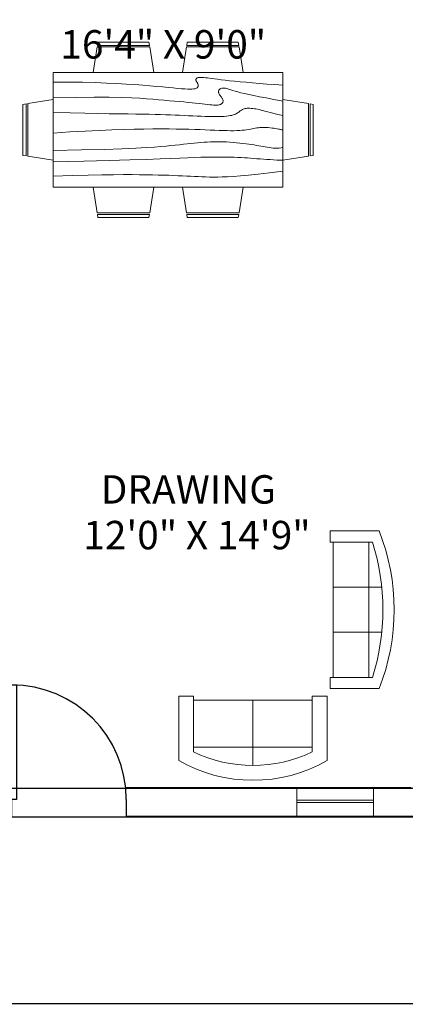
# Model space of a CAD drawing. Units: inches. Extents: x -46 to 1145, y -527 to 760.
# Tile 18 of 57: x 788 to 909, y -527 to -218. Entities that reach past the tile are written whole.
import ezdxf

# ---------------------------------------------------------------- set-up
doc = ezdxf.new("R2010")
doc.units = ezdxf.units.IN
doc.header["$MEASUREMENT"] = 0
for name, color, linetype, lineweight in [('A-ANNO-DIMS', 2, 'Continuous', 18), ('A-AREA-IDEN', 1, 'Continuous', 18), ('A-FURN', 2, 'Continuous', 13), ('C-SITE', 7, 'Continuous', 30), ('DOORS', 3, 'Continuous', 25), ('WALLS', 4, 'Continuous', 40), ('WINDOWS', 240, 'Continuous', 20)]:
    doc.layers.add(name, color=color, linetype=linetype, lineweight=lineweight)
doc.styles.get("Standard").update_dxf_attribs({"font": 'arial.ttf'})
doc.dimstyles.get("Standard").update_dxf_attribs({"dimtxt": 0.18, "dimasz": 0.18, "dimexe": 0.18, "dimexo": 0.0625, "dimgap": 0.09, "dimtad": 0, "dimtih": 1, "dimtoh": 1, "dimdec": 0, "dimzin": 0, "dimdsep": 46, "dimlunit": 3, "dimtxsty": 'Standard', "dimcen": 0.09, "dimadec": 0, "dimazin": 0, "dimtfac": 1, "dimtdec": 0, "dimtofl": 0, "dimtmove": 0, "dimatfit": 3, "dimfxl": 1, "dimtolj": 1, "dimtzin": 0, "dimarcsym": 0})

# ---------------------------------------------------------------- blocks, each defined once
blk = doc.blocks.new('Dining Set - 36 x 72 in.')
for p, q in [((-22.2343, 26.00059), (-23.4847, 17.99762)), ((-22.2304, 26), (-5.7608, 26)), ((-22, 27.5), (-22.1562, 26.50042)), ((-5.8416, 26.5), (-22.1534, 26.5)), ((-22, 27.5), (-6, 27.5)), ((-5.8437, 26.49966), (-6, 27.5)), ((-4.5152, 17.99762), (-5.7655, 25.99926)), ((5.7657, 26.00059), (4.5153, 17.99762)), ((5.7696, 26), (22.2392, 26)), ((6, 27.5), (5.8438, 26.50042)), ((22.1584, 26.5), (5.8466, 26.5)), ((6, 27.5), (22, 27.5)), ((22.1563, 26.49966), (22, 27.5)), ((23.4848, 17.99762), (22.2345, 25.99926)), ((36, 18), (-36, 18)), ((-36, 18), (-36, -18)), ((36, -18), (36, 18)), ((-44.0006, 8.23428), (-35.9976, 9.48474)), ((44.0006, 8.23428), (35.9976, 9.48474)), ((-45.5, 8), (-44.5004, 8.15617)), ((-45.5, 8), (-45.5, -8)), ((-44.5, -8.15843), (-44.5, 8.15338)), ((-44, 8.23041), (-44, -8.23915)), ((44, 8.23041), (44, -8.23915)), ((44.5, -8.15843), (44.5, 8.15338)), ((45.5, 8), (44.5005, 8.15617)), ((45.5, 8), (45.5, -8)), ((-44.4997, -8.15631), (-45.5, -8)), ((-35.9976, -9.48476), (-43.9993, -8.2345)), ((35.9976, -9.48476), (43.9993, -8.2345)), ((44.4997, -8.15631), (45.5, -8)), ((-36, -18), (36, -18)), ((-22.2343, -26.0006), (-23.4847, -17.99762)), ((-4.5152, -17.99762), (-5.7655, -25.99928)), ((5.7657, -26.0006), (4.5153, -17.99762)), ((23.4848, -17.99762), (22.2345, -25.99928)), ((-22.2304, -26), (-5.7608, -26)), ((-22, -27.5), (-22.1562, -26.50044)), ((-5.8416, -26.5), (-22.1534, -26.5)), ((-22, -27.5), (-6, -27.5)), ((-5.8437, -26.49967), (-6, -27.5)), ((5.7696, -26), (22.2392, -26)), ((6, -27.5), (5.8438, -26.50044)), ((22.1584, -26.5), (5.8466, -26.5)), ((6, -27.5), (22, -27.5)), ((22.1563, -26.49967), (22, -27.5))]:
    blk.add_line(p, q)
for points in [[(-36, 15), (-31.1772, 14.97754), (-26.8079, 14.91406), (-22.8538, 14.81543), (-19.276, 14.6875), (-16.0362, 14.53613), (-13.0957, 14.36718), (-10.4159, 14.18652), (-7.9583, 14), (-5.6904, 13.81315), (-3.6035, 13.63021), (-1.6954, 13.45508), (0.0365, 13.29166), (1.5945, 13.14388), (2.9811, 13.01562), (4.1988, 12.9108), (5.25, 12.83333), (6.1393, 12.78613), (6.8802, 12.76823), (7.4883, 12.77767), (7.9792, 12.8125), (8.3685, 12.87077), (8.6719, 12.95052), (8.9049, 13.0498), (9.0833, 13.16666), (9.2205, 13.29899), (9.3216, 13.44401), (9.3895, 13.59879), (9.4271, 13.76041), (9.4373, 13.92594), (9.4232, 14.09245), (9.3875, 14.257), (9.3333, 14.41666), (9.2638, 14.56917), (9.1836, 14.71484), (9.0975, 14.85465), (9.0104, 14.98958), (8.9272, 15.1206), (8.8529, 15.2487), (8.7922, 15.37483), (8.75, 15.5), (8.7305, 15.62467), (8.7344, 15.74739), (8.7617, 15.86621), (8.8125, 15.97916), (8.8867, 16.08431), (8.9844, 16.17968), (9.1055, 16.26334), (9.25, 16.33333), (9.4189, 16.38802), (9.6172, 16.42708), (9.8506, 16.45052), (10.125, 16.45833), (10.4463, 16.45052), (10.8203, 16.42708), (11.2529, 16.38802), (11.75, 16.33333), (12.3184, 16.26318), (12.9694, 16.17838), (13.7151, 16.07991), (14.5677, 15.96875), (15.5395, 15.84586), (16.6426, 15.71224), (17.8893, 15.56884), (19.2917, 15.41666), (20.859, 15.25667), (22.5879, 15.08984), (24.4721, 14.91715), (26.5052, 14.73958), (28.6809, 14.5581), (30.9929, 14.3737), (33.4347, 14.18733), (36, 14)], [(-36, 10), (-28.9766, 10.14274), (-23.1725, 10.20442), (-18.4241, 10.19775), (-14.5677, 10.13541), (-11.4399, 10.03011), (-8.877, 9.89453), (-6.7154, 9.74137), (-4.7917, 9.58333), (-2.9698, 9.43082), (-1.2246, 9.28515), (0.4415, 9.14534), (2.026, 9.01041), (3.5266, 8.87939), (4.9408, 8.7513), (6.266, 8.62516), (7.5, 8.5), (8.6411, 8.37549), (9.6914, 8.2539), (10.6538, 8.13818), (11.5312, 8.03125), (12.3267, 7.93603), (13.043, 7.85547), (13.6831, 7.79248), (14.25, 7.75), (14.7471, 7.7303), (15.1797, 7.73307), (15.5537, 7.75732), (15.875, 7.80208), (16.1494, 7.86637), (16.3828, 7.94922), (16.5811, 8.04964), (16.75, 8.16666), (16.8944, 8.29915), (17.0143, 8.44531), (17.1089, 8.60319), (17.1771, 8.77083), (17.218, 8.94629), (17.2305, 9.1276), (17.2137, 9.31282), (17.1667, 9.5), (17.0895, 9.6875), (16.987, 9.875), (16.8649, 10.0625), (16.7292, 10.25), (16.5856, 10.4375), (16.4401, 10.625), (16.2985, 10.8125), (16.1667, 11), (16.05, 11.18733), (15.9518, 11.3737), (15.8752, 11.5581), (15.8229, 11.73958), (15.798, 11.91715), (15.8034, 12.08984), (15.842, 12.25667), (15.9167, 12.41666), (16.0295, 12.56836), (16.1784, 12.70833), (16.3605, 12.83268), (16.5729, 12.9375), (16.8127, 13.01888), (17.0768, 13.07291), (17.3625, 13.0957), (17.6667, 13.08333), (17.9894, 13.03312), (18.3418, 12.94726), (18.7382, 12.82918), (19.1927, 12.68229), (19.7195, 12.51001), (20.3327, 12.31575), (21.0465, 12.10294), (21.875, 11.875), (22.8357, 11.63354), (23.959, 11.37304), (25.2786, 11.08618), (26.8282, 10.76562), (28.6414, 10.40405), (30.752, 9.99414), (33.1936, 9.52856), (36, 9)], [(-36, 5.5), (-30.7157, 5.3348), (-26.069, 5.20963), (-21.9946, 5.11767), (-18.4271, 5.05208), (-15.3009, 5.00602), (-12.5508, 4.97265), (-10.1112, 4.94515), (-7.9167, 4.91666), (-5.909, 4.88167), (-4.0586, 4.83984), (-2.3429, 4.79215), (-0.7396, 4.73958), (0.7739, 4.6831), (2.22, 4.6237), (3.6213, 4.56233), (5, 4.5), (6.373, 4.43782), (7.7344, 4.3776), (9.0723, 4.32129), (10.375, 4.27083), (11.6309, 4.22819), (12.8281, 4.19531), (13.9551, 4.17415), (15, 4.16666), (15.954, 4.17448), (16.819, 4.19791), (17.6001, 4.23698), (18.3021, 4.29166), (18.9299, 4.36198), (19.4883, 4.44791), (19.9823, 4.54948), (20.4167, 4.66666), (20.7969, 4.79899), (21.1302, 4.94401), (21.4245, 5.09879), (21.6875, 5.26041), (21.9271, 5.42594), (22.1511, 5.59245), (22.3672, 5.757), (22.5834, 5.91666), (22.8065, 6.06868), (23.0404, 6.21093), (23.2879, 6.34147), (23.5521, 6.45833), (23.8358, 6.55957), (24.142, 6.64323), (24.4735, 6.70735), (24.8334, 6.75), (25.2235, 6.76969), (25.642, 6.76692), (26.0858, 6.74267), (26.5521, 6.69791), (27.0379, 6.63362), (27.5404, 6.55078), (28.0565, 6.45036), (28.5834, 6.33333), (29.1242, 6.19987), (29.7071, 6.04687), (30.3661, 5.87044), (31.1354, 5.66666), (32.0493, 5.43164), (33.142, 5.16146), (34.4475, 4.85221), (36, 4.5)], [(-36, -1), (-30.7915, -0.6591), (-26.0195, -0.38216), (-21.6519, -0.16284), (-17.6563, 0.00521), (-14.0005, 0.12833), (-10.6523, 0.21289), (-7.5796, 0.26522), (-4.75, 0.29166), (-2.134, 0.29793), (0.2878, 0.28711), (2.5317, 0.26163), (4.6146, 0.22396), (6.5529, 0.17651), (8.3633, 0.12174), (10.0623, 0.06209), (11.6667, 0), (13.1899, -0.06201), (14.6341, -0.1211), (15.9982, -0.17432), (17.2813, -0.21875), (18.4823, -0.25147), (19.6003, -0.26953), (20.6343, -0.27002), (21.5834, -0.25), (22.4481, -0.20768), (23.2357, -0.14584), (23.9549, -0.06836), (24.6146, 0.02083), (25.2235, 0.11784), (25.7904, 0.21875), (26.3241, 0.31966), (26.8334, 0.41666), (27.3265, 0.50618), (27.8099, 0.58593), (28.2894, 0.65397), (28.7709, 0.70833), (29.2601, 0.74707), (29.763, 0.76823), (30.2855, 0.76985), (30.8334, 0.75), (31.4088, 0.70784), (31.9994, 0.64713), (32.589, 0.57275), (33.1615, 0.48958), (33.7008, 0.4025), (34.1908, 0.3164), (34.6153, 0.23616), (34.9584, 0.16666), (35.2099, 0.11165), (35.3848, 0.07031), (35.504, 0.04069), (35.5886, 0.02083), (35.6594, 0.00879), (35.7377, 0.0026), (35.8442, 0.00032), (36, 0)], [(-36, -6.5), (-27.1843, -6.31267), (-20.084, -6.1263), (-14.469, -5.9419), (-10.1094, -5.76042), (-6.7752, -5.58285), (-4.2363, -5.41016), (-2.2629, -5.24333), (-0.625, -5.08334), (0.8708, -4.93099), (2.2715, -4.78646), (3.5872, -4.64974), (4.8281, -4.52084), (6.0046, -4.39974), (7.127, -4.28646), (8.2053, -4.18099), (9.25, -4.08334), (10.2705, -3.99382), (11.2734, -3.91407), (12.2647, -3.84603), (13.25, -3.79167), (14.2354, -3.75293), (15.2266, -3.73177), (16.2295, -3.73015), (17.25, -3.75), (18.2912, -3.79248), (19.3451, -3.85547), (20.4009, -3.93604), (21.4479, -4.03125), (22.4754, -4.13819), (23.4727, -4.25391), (24.4289, -4.37549), (25.3334, -4.5), (26.1785, -4.62492), (26.9694, -4.74935), (27.7145, -4.87281), (28.4219, -4.99479), (29.1, -5.11483), (29.7572, -5.23242), (30.4016, -5.34709), (31.0417, -5.45834), (31.6837, -5.56437), (32.3262, -5.65821), (32.9658, -5.73153), (33.599, -5.77604), (34.2224, -5.78345), (34.8327, -5.74545), (35.4264, -5.65373), (36, -5.5)], [(-36, -10), (-26.4022, -9.81299), (-18.4675, -9.62891), (-11.9839, -9.45069), (-6.7396, -9.28125), (-2.5226, -9.12354), (0.8789, -8.98047), (3.6769, -8.85498), (6.0833, -8.75), (8.2767, -8.66765), (10.3021, -8.60677), (12.1712, -8.56543), (13.8958, -8.54167), (15.4876, -8.53353), (16.9583, -8.53907), (18.3197, -8.55632), (19.5834, -8.58334), (20.7616, -8.61841), (21.8685, -8.66081), (22.9188, -8.71004), (23.9271, -8.76563), (24.9081, -8.82707), (25.8763, -8.89388), (26.8465, -8.96558), (27.8334, -9.04167), (28.8474, -9.12118), (29.8828, -9.20117), (30.93, -9.27824), (31.9792, -9.34896), (33.0205, -9.40991), (34.0443, -9.45768), (35.0407, -9.48885), (36, -9.5)], [(-36, -14.5), (-30.0881, -14.33513), (-25.0332, -14.21224), (-20.7312, -14.12647), (-17.0781, -14.07292), (-13.97, -14.04671), (-11.3027, -14.04297), (-8.9724, -14.05681), (-6.875, -14.08334), (-4.9224, -14.11833), (-3.0905, -14.16016), (-1.3709, -14.20785), (0.2448, -14.26042), (1.7647, -14.3169), (3.1973, -14.3763), (4.5507, -14.43767), (5.8333, -14.5), (7.0554, -14.5621), (8.235, -14.62175), (9.3922, -14.67652), (10.5469, -14.72396), (11.7192, -14.76164), (12.929, -14.78711), (14.1965, -14.79794), (15.5417, -14.79167), (16.9933, -14.76424), (18.6152, -14.70508), (20.4804, -14.60197), (22.6615, -14.44271), (25.2312, -14.21509), (28.2624, -13.9069), (31.8277, -13.50594), (36, -13)]]:
    blk.add_lwpolyline(points)
blk = doc.blocks.new('Sofa - Roundback 7 ft.')
for p, q in [((-12.00002, -32.4421), (-12.00003, -6.5971)), ((11.99997, -32.4421), (11.99998, -6.5971)), ((-36.000027, -34), (-36.000027, -11.4696)), ((-35.999844, -13.3819), (35.9998, -13.3819)), ((35.99998, -34), (35.99998, -11.4696)), ((-36.000027, -32.4421), (35.99998, -32.4421))]:
    blk.add_line(p, q)
for points in [[(-36.000027, -34), (-42.000027, -34), (-42.000027, -8)], [(41.99998, -8), (41.99998, -34), (35.99998, -34)]]:
    blk.add_lwpolyline(points)
for centre, radius, start, end in [((0, -114.25), 114.25, 68.43141, 111.5686), ((-0.00001, -127.1968), 121.1968, 72.72033, 107.2797)]:
    blk.add_arc(centre, radius, start, end)
blk = doc.blocks.new('Sofa - Roundback Loveseat 5 ft.')
for p, q in [((0, -32.44198), (0, -5.99998)), ((-24, -33.99998), (-24, -11.46958)), ((24.00004, -33.99998), (24.00004, -11.46958)), ((-23.9998, -13.38178), (23.99986, -13.38178)), ((-24, -32.44198), (24.00004, -32.44198))]:
    blk.add_line(p, q)
for points in [[(-24, -33.99998), (-30, -33.99998), (-30, -7.99998)], [(30.00004, -7.99998), (30.00004, -33.99998), (24.00004, -33.99998)]]:
    blk.add_lwpolyline(points)
for centre, radius, start, end in [((0, -60.24998), 60.24998, 60.13715, 119.8628), ((0, -61.38438), 55.38444, 64.32083, 115.6792)]:
    blk.add_arc(centre, radius, start, end)
blk = doc.blocks.new('*U2')
for p, q in [((0, 0), (0, -6)), ((40, 0), (40, -6))]:
    blk.add_line(p, q)
blk.add_lwpolyline([(0, 0), (0, 40), (1.75, 40), (1.75, 0)], close=True)
blk.add_arc((0, 0), 40, 0, 90)
blk = doc.blocks.new('WINDOW-24IN')
for p, q in [((0, 4.5), (0, 9)), ((0, 9), (0, 0)), ((24, 9), (24, 0)), ((0, 5.23), (24, 5.23)), ((0, 4.5), (24, 4.5))]:
    blk.add_line(p, q)
blk = doc.blocks.new('*D684')
at = {"layer": 'A-ANNO-DIMS', "color": 0, "lineweight": -2, "transparency": 16777216}
for p, q in [((12.56, -468.54), (12.56, -527.26)), ((1086.56, -468.54), (1086.56, -527.26)), ((12.74, -527.08), (549.21, -527.08)), ((1086.38, -527.08), (549.91, -527.08))]:
    blk.add_line(p, q, dxfattribs=at)
at = {"layer": 'A-ANNO-DIMS', "color": 0, "transparency": 16777216}
for points in [[(12.74, -527.05), (12.74, -527.11), (12.56, -527.08)], [(1086.38, -527.05), (1086.38, -527.11), (1086.56, -527.08)]]:
    blk.add_solid(points, dxfattribs=at)
at = {"layer": 'Defpoints', "color": 0, "transparency": 16777216}
for p in [(12.56, -468.48), (1086.56, -468.48), (1086.56, -527.08)]:
    blk.add_point(p, dxfattribs=at)
at = {"layer": 'A-ANNO-DIMS', "color": 0, "transparency": 16777216, "insert": (549.56, -527.08), "char_height": 0.18, "attachment_point": 5}
blk.add_mtext('\\A1;1074', dxfattribs=at)
blk = doc.blocks.new('*D702')
at = {"layer": 'A-ANNO-DIMS', "color": 0, "lineweight": -2, "transparency": 16777216}
for p, q in [((189.63, -39.48), (1145.34, -39.48)), ((1145.16, -39.66), (1145.16, -249.3)), ((1145.16, -459.3), (1145.16, -249.66)), ((183.63, -459.48), (1145.34, -459.48))]:
    blk.add_line(p, q, dxfattribs=at)
at = {"layer": 'A-ANNO-DIMS', "color": 0, "transparency": 16777216}
for points in [[(1145.13, -39.66), (1145.19, -39.66), (1145.16, -39.48)], [(1145.13, -459.3), (1145.19, -459.3), (1145.16, -459.48)]]:
    blk.add_solid(points, dxfattribs=at)
at = {"layer": 'Defpoints', "color": 0, "transparency": 16777216}
for p in [(189.56, -39.48), (1145.16, -39.48), (183.56, -459.48)]:
    blk.add_point(p, dxfattribs=at)
at = {"layer": 'A-ANNO-DIMS', "color": 0, "transparency": 16777216, "insert": (1145.16, -249.48), "char_height": 0.18, "attachment_point": 5}
blk.add_mtext('\\A1;420', dxfattribs=at)

msp = doc.modelspace()

# ---------------------------------------------------------------- linework, layer by layer
at = {"layer": 'C-SITE'}
for p, q in [((21.5637, -459.4824), (1077.5637, -459.4824)), ((12.5637, -468.4824), (1086.5637, -468.4824))]:
    msp.add_line(p, q, dxfattribs=at)
at = {"layer": 'WALLS'}
for p, q in [((911.0637, -459.4824), (821.5926, -459.4824)), ((1086.5637, -468.4824), (821.7731, -468.4824))]:
    msp.add_line(p, q, dxfattribs=at)

# ---------------------------------------------------------------- block references
at = {"layer": 'A-FURN'}
msp.add_blockref('Dining Set - 36 x 72 in.', (834.8617, -253.0428), dxfattribs=at)
for name, p, xscale, yscale, zscale, rotation in [('Sofa - Roundback 7 ft.', (905.7179, -403.5162), 0.5892128430585409, 0.5892128430585409, 0.5892128430585409, 270), ('Sofa - Roundback Loveseat 5 ft.', (861.4562, -457.0139), 0.7756934806711657, 0.7756934806711657, 0.7756934806711657, 180)]:
    msp.add_blockref(name, p, dxfattribs=dict(at, xscale=xscale, yscale=yscale, zscale=zscale, rotation=rotation))
at = {"layer": 'DOORS', "xscale": 0.9, "yscale": 0.9, "zscale": 0.9}
msp.add_blockref('*U2', (785.7731, -463.0824), dxfattribs=at)
at = {"layer": 'WINDOWS'}
msp.add_blockref('WINDOW-24IN', (875.233, -468.482), dxfattribs=at)

# ---------------------------------------------------------------- texts
at = {"layer": 'A-AREA-IDEN'}
for s, height, p in [('16\'4" X 9\'0"', 8.923264, (801.1059, -230.6935)), ('  DRAWING', 8.92326, (808.2854, -370.2544)), ('12\'0" X 14\'9"', 8.923264, (808.2854, -384.5888))]:
    msp.add_text(s, height=height, dxfattribs=at).set_placement(p)

# ---------------------------------------------------------------- dimensions: what is measured, and where the dimension line sits
at = {"layer": 'A-ANNO-DIMS'}
dim = msp.add_linear_dim(base=(1145.1637, -39.4824), p1=(183.5637, -459.4824), p2=(189.5637, -39.4824), angle=90, dimstyle='Standard', override={"dimdec": 0, "dimlfac": 1, "dimrnd": 0, "dimzin": 0, "dimdsep": 46, "dimlunit": 2}, dxfattribs=at)
dim.commit()
dim.dimension.update_dxf_attribs({"geometry": '*D702', "text_midpoint": (1145.1637, -249.4824)})
dim = msp.add_linear_dim(base=(1086.5637, -527.0824), p1=(12.5637, -468.4824), p2=(1086.5637, -468.4824), dimstyle='Standard', override={"dimdec": 0, "dimlfac": 1, "dimrnd": 0, "dimzin": 0, "dimdsep": 46, "dimlunit": 2}, dxfattribs=at)
dim.commit()
dim.dimension.update_dxf_attribs({"geometry": '*D684', "text_midpoint": (549.5637, -527.0824)})

doc.saveas('drawing.dxf')
